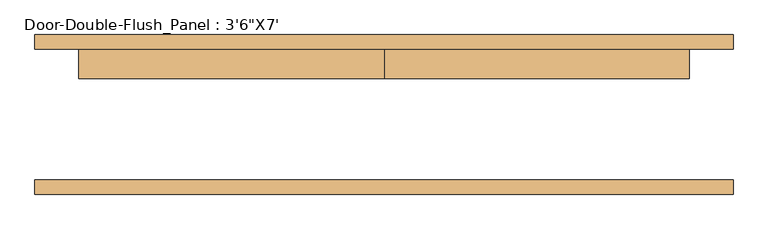
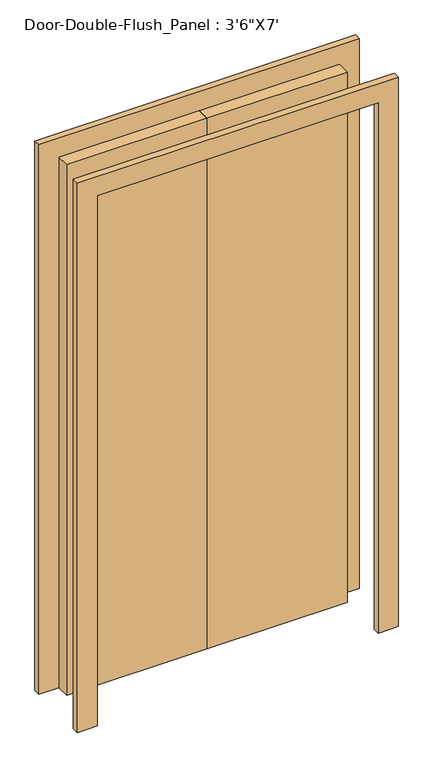
"""IFC4 building model written with IfcOpenShell, lengths in millimetres: door geometry."""

from ifc_helpers import new_model, si_unit, frame, origin, origin_with_axes, place, context, project, spatial, polyline, outline, extrude, source, transform, mapped, element, save


def door_d52489d9(model_context):
    return source(origin(), model_context, "Body", "SweptSolid", [
        extrude(outline(polyline([(2133.6, -533.4), (2133.6, 533.4), (0.0, 533.4), (0.0, 609.6), (2209.8, 609.6), (2209.8, -609.6), (0.0, -609.6), (0.0, -533.4), (2133.6, -533.4)])), frame((0.0, 114.3, 0.0), z_axis=(0.0, 1.0, 0.0), x_axis=(0.0, 0.0, 1.0)), (0.0, 0.0, 1.0), 25.4),
        extrude(outline(polyline([(2133.6, -533.4), (2133.6, 533.4), (0.0, 533.4), (0.0, 609.6), (2209.8, 609.6), (2209.8, -609.6), (0.0, -609.6), (0.0, -533.4), (2133.6, -533.4)])), frame((0.0, -139.7, 0.0), z_axis=(0.0, 1.0, 0.0), x_axis=(0.0, 0.0, 1.0)), (0.0, 0.0, 1.0), 25.4),
        extrude(outline(polyline([(-533.4, 114.3), (0.0, 114.3), (0.0, 63.5), (-533.4, 63.5), (-533.4, 114.3)])), origin_with_axes(), (0.0, 0.0, 1.0), 2133.6),
        extrude(outline(polyline([(0.0, 114.3), (533.4, 114.3), (533.4, 63.5), (0.0, 63.5), (0.0, 114.3)])), origin_with_axes(), (0.0, 0.0, 1.0), 2133.6),
    ])


if __name__ == "__main__":
    model = new_model("IFC4")
    model_context = context("Model", 3, world=origin())
    ifc_project = project(units=[si_unit("LENGTHUNIT", "METRE", prefix="MILLI")], contexts=[model_context])
    site = spatial("IfcSite", under=ifc_project)
    building = spatial("IfcBuilding", under=site)
    placement = place(None, origin())
    door_shape = door_d52489d9(model_context)
    element("IfcDoor", 1, ObjectType="Door-Double-Flush_Panel : 3'6\"X7'", at=placement, inside=building, context=model_context, shape_type="MappedRepresentation", body=[
        mapped(door_shape, transform((0.0, 0.0, 0.0), x_axis=(1.0, 0.0, 0.0), y_axis=(0.0, 1.0, 0.0), z_axis=(0.0, 0.0, 1.0))),
    ])
    save(model, "model.ifc")

# Revit data of these elements
# Type "Door-Double-Flush_Panel : 3'6\"X7'"
#   Type Mark = "12"
#   Construction Type Id = "DOOR"
#   Assembly Code = "C1020"
#   Analytic Construction = "Wooden"
#   Thickness = 0' - 2"
#   Thermal Resistance (R) = 2.5876 (h·ft²·°F)/BTU
#   Swing Angle [instance default] = 90.00°
#   Panel Width = 1' - 9"
#   Heat Transfer Coefficient (U) = 0.3865 BTU/(h·ft²·°F)
#   Height = 7' - 0"
#   Trim Projection Ext = 0' - 1"
#   Trim Projection Int = 0' - 1"
#   Trim Width = 0' - 3"
#   Width = 3' - 6"
#   Define Thermal Properties by = 1
#   Panel Material = Wood - Birch - Solid Stained Light Low Gloss
#   Trim Material = Paint - Sienna
#   Visual Light Transmittance = 0
#   Solar Heat Gain Coefficient = 0
#   Function = (empty or 0)
#   Wall Closure = (empty or 0)
# Element 1 (IfcDoor, "Door-Double-Flush_Panel : 3'6\"X7'")
#   Materials on its faces: "Paint - Sienna", "Wood - Birch - Solid Stained Light Low Gloss"
# Materials
#   "Wood - Birch - Solid Stained Light Low Gloss": class "Wood", colour RGB 210 159 95, transparency 0, Cost = 0
#   "Paint - Sienna": colour RGB 118 70 51, transparency 0, Cost = 0
